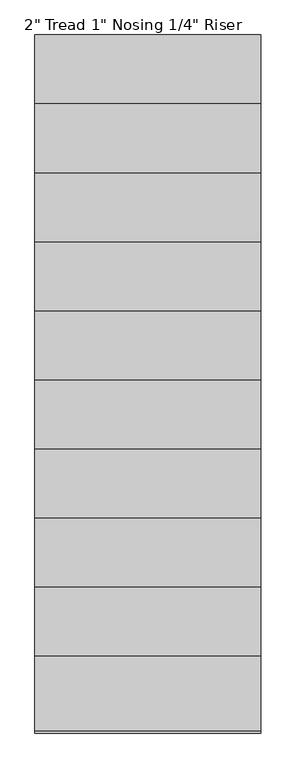
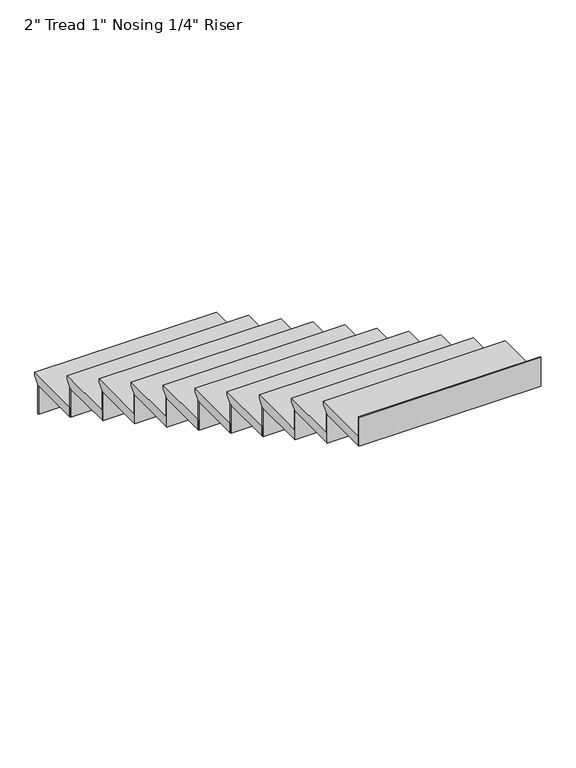
"""IFC4 building model written with IfcOpenShell, lengths in millimetres: stair flight geometry."""

from ifc_helpers import new_model, si_unit, frame, origin, place, context, project, spatial, polyline, outline, extrude, source, transform, mapped, element, save


def stair_flight_b2a94bac(model_context):
    return source(origin(), model_context, "Body", "SweptSolid", [
        extrude(outline(polyline([(4154.8726898, 1524.0), (4459.6726898, 1524.0), (4459.6726898, 1504.95), (4434.2726898, 1479.55), (4434.2726898, 1473.2), (4154.8726898, 1473.2), (4154.8726898, 1524.0)])), frame((1247.5463194, 0.0, 0.0), z_axis=(1.0, 0.0, 0.0), x_axis=(0.0, 1.0, 0.0)), (0.0, 0.0, 1.0), 914.4),
        extrude(outline(polyline([(1247.5463194, 4427.9226898), (1247.5463194, 4434.2726898), (2161.9463194, 4434.2726898), (2161.9463194, 4427.9226898), (1247.5463194, 4427.9226898)])), frame((0.0, 0.0, 1320.8), z_axis=(0.0, 0.0, 1.0), x_axis=(1.0, 0.0, 0.0)), (0.0, 0.0, 1.0), 152.4),
        extrude(outline(polyline([(1247.5463194, 4148.5226898), (1247.5463194, 4154.8726898), (2161.9463194, 4154.8726898), (2161.9463194, 4148.5226898), (1247.5463194, 4148.5226898)])), frame((0.0, 0.0, 1473.2), z_axis=(0.0, 0.0, 1.0), x_axis=(1.0, 0.0, 0.0)), (0.0, 0.0, 1.0), 152.4),
        extrude(outline(polyline([(3875.4726898, 1676.4), (4180.2726898, 1676.4), (4180.2726898, 1657.35), (4154.8726898, 1631.95), (4154.8726898, 1625.6), (3875.4726898, 1625.6), (3875.4726898, 1676.4)])), frame((1247.5463194, 0.0, 0.0), z_axis=(1.0, 0.0, 0.0), x_axis=(0.0, 1.0, 0.0)), (0.0, 0.0, 1.0), 914.4),
        extrude(outline(polyline([(1247.5463194, 3869.1226898), (1247.5463194, 3875.4726898), (2161.9463194, 3875.4726898), (2161.9463194, 3869.1226898), (1247.5463194, 3869.1226898)])), frame((0.0, 0.0, 1625.6), z_axis=(0.0, 0.0, 1.0), x_axis=(1.0, 0.0, 0.0)), (0.0, 0.0, 1.0), 152.4),
        extrude(outline(polyline([(3596.0726898, 1828.8), (3900.8726898, 1828.8), (3900.8726898, 1809.75), (3875.4726898, 1784.35), (3875.4726898, 1778.0), (3596.0726898, 1778.0), (3596.0726898, 1828.8)])), frame((1247.5463194, 0.0, 0.0), z_axis=(1.0, 0.0, 0.0), x_axis=(0.0, 1.0, 0.0)), (0.0, 0.0, 1.0), 914.4),
        extrude(outline(polyline([(1247.5463194, 3589.7226898), (1247.5463194, 3596.0726898), (2161.9463194, 3596.0726898), (2161.9463194, 3589.7226898), (1247.5463194, 3589.7226898)])), frame((0.0, 0.0, 1778.0), z_axis=(0.0, 0.0, 1.0), x_axis=(1.0, 0.0, 0.0)), (0.0, 0.0, 1.0), 152.4),
        extrude(outline(polyline([(3316.6726898, 1981.2), (3621.4726898, 1981.2), (3621.4726898, 1962.15), (3596.0726898, 1936.75), (3596.0726898, 1930.4), (3316.6726898, 1930.4), (3316.6726898, 1981.2)])), frame((1247.5463194, 0.0, 0.0), z_axis=(1.0, 0.0, 0.0), x_axis=(0.0, 1.0, 0.0)), (0.0, 0.0, 1.0), 914.4),
        extrude(outline(polyline([(1247.5463194, 3310.3226898), (1247.5463194, 3316.6726898), (2161.9463194, 3316.6726898), (2161.9463194, 3310.3226898), (1247.5463194, 3310.3226898)])), frame((0.0, 0.0, 1930.4), z_axis=(0.0, 0.0, 1.0), x_axis=(1.0, 0.0, 0.0)), (0.0, 0.0, 1.0), 152.4),
        extrude(outline(polyline([(3037.2726898, 2133.6), (3342.0726898, 2133.6), (3342.0726898, 2114.55), (3316.6726898, 2089.15), (3316.6726898, 2082.8), (3037.2726898, 2082.8), (3037.2726898, 2133.6)])), frame((1247.5463194, 0.0, 0.0), z_axis=(1.0, 0.0, 0.0), x_axis=(0.0, 1.0, 0.0)), (0.0, 0.0, 1.0), 914.4),
        extrude(outline(polyline([(1247.5463194, 3030.9226898), (1247.5463194, 3037.2726898), (2161.9463194, 3037.2726898), (2161.9463194, 3030.9226898), (1247.5463194, 3030.9226898)])), frame((0.0, 0.0, 2082.8), z_axis=(0.0, 0.0, 1.0), x_axis=(1.0, 0.0, 0.0)), (0.0, 0.0, 1.0), 152.4),
        extrude(outline(polyline([(2757.8726898, 2286.0), (3062.6726898, 2286.0), (3062.6726898, 2266.95), (3037.2726898, 2241.55), (3037.2726898, 2235.2), (2757.8726898, 2235.2), (2757.8726898, 2286.0)])), frame((1247.5463194, 0.0, 0.0), z_axis=(1.0, 0.0, 0.0), x_axis=(0.0, 1.0, 0.0)), (0.0, 0.0, 1.0), 914.4),
        extrude(outline(polyline([(1247.5463194, 2751.5226898), (1247.5463194, 2757.8726898), (2161.9463194, 2757.8726898), (2161.9463194, 2751.5226898), (1247.5463194, 2751.5226898)])), frame((0.0, 0.0, 2235.2), z_axis=(0.0, 0.0, 1.0), x_axis=(1.0, 0.0, 0.0)), (0.0, 0.0, 1.0), 152.4),
        extrude(outline(polyline([(2478.4726898, 2438.4), (2783.2726898, 2438.4), (2783.2726898, 2419.35), (2757.8726898, 2393.95), (2757.8726898, 2387.6), (2478.4726898, 2387.6), (2478.4726898, 2438.4)])), frame((1247.5463194, 0.0, 0.0), z_axis=(1.0, 0.0, 0.0), x_axis=(0.0, 1.0, 0.0)), (0.0, 0.0, 1.0), 914.4),
        extrude(outline(polyline([(1247.5463194, 2472.1226898), (1247.5463194, 2478.4726898), (2161.9463194, 2478.4726898), (2161.9463194, 2472.1226898), (1247.5463194, 2472.1226898)])), frame((0.0, 0.0, 2387.6), z_axis=(0.0, 0.0, 1.0), x_axis=(1.0, 0.0, 0.0)), (0.0, 0.0, 1.0), 152.4),
        extrude(outline(polyline([(2199.0726898, 2590.8), (2503.8726898, 2590.8), (2503.8726898, 2571.75), (2478.4726898, 2546.35), (2478.4726898, 2540.0), (2199.0726898, 2540.0), (2199.0726898, 2590.8)])), frame((1247.5463194, 0.0, 0.0), z_axis=(1.0, 0.0, 0.0), x_axis=(0.0, 1.0, 0.0)), (0.0, 0.0, 1.0), 914.4),
        extrude(outline(polyline([(1247.5463194, 2192.7226898), (1247.5463194, 2199.0726898), (2161.9463194, 2199.0726898), (2161.9463194, 2192.7226898), (1247.5463194, 2192.7226898)])), frame((0.0, 0.0, 2540.0), z_axis=(0.0, 0.0, 1.0), x_axis=(1.0, 0.0, 0.0)), (0.0, 0.0, 1.0), 152.4),
        extrude(outline(polyline([(1919.6726898, 2743.2), (2224.4726898, 2743.2), (2224.4726898, 2724.15), (2199.0726898, 2698.75), (2199.0726898, 2692.4), (1919.6726898, 2692.4), (1919.6726898, 2743.2)])), frame((1247.5463194, 0.0, 0.0), z_axis=(1.0, 0.0, 0.0), x_axis=(0.0, 1.0, 0.0)), (0.0, 0.0, 1.0), 914.4),
        extrude(outline(polyline([(1247.5463194, 1913.3226898), (1247.5463194, 1919.6726898), (2161.9463194, 1919.6726898), (2161.9463194, 1913.3226898), (1247.5463194, 1913.3226898)])), frame((0.0, 0.0, 2692.4), z_axis=(0.0, 0.0, 1.0), x_axis=(1.0, 0.0, 0.0)), (0.0, 0.0, 1.0), 152.4),
        extrude(outline(polyline([(1247.5463194, 1633.9226898), (1247.5463194, 1640.2726898), (2161.9463194, 1640.2726898), (2161.9463194, 1633.9226898), (1247.5463194, 1633.9226898)])), frame((0.0, 0.0, 2844.8), z_axis=(0.0, 0.0, 1.0), x_axis=(1.0, 0.0, 0.0)), (0.0, 0.0, 1.0), 152.4),
        extrude(outline(polyline([(1640.2726898, 2895.6), (1945.0726898, 2895.6), (1945.0726898, 2876.55), (1919.6726898, 2851.15), (1919.6726898, 2844.8), (1640.2726898, 2844.8), (1640.2726898, 2895.6)])), frame((1247.5463194, 0.0, 0.0), z_axis=(1.0, 0.0, 0.0), x_axis=(0.0, 1.0, 0.0)), (0.0, 0.0, 1.0), 914.4),
    ])


if __name__ == "__main__":
    model = new_model("IFC4")
    model_context = context("Model", 3, world=origin())
    ifc_project = project(units=[si_unit("LENGTHUNIT", "METRE", prefix="MILLI")], contexts=[model_context])
    site = spatial("IfcSite", under=ifc_project)
    building = spatial("IfcBuilding", under=site)
    placement = place(None, origin())
    stair_flight_shape = stair_flight_b2a94bac(model_context)
    element("IfcStairFlight", 1, ObjectType="2\" Tread 1\" Nosing 1/4\" Riser", at=placement, inside=building, context=model_context, shape_type="MappedRepresentation", body=[
        mapped(stair_flight_shape, transform((0.0, 0.0, 0.0), x_axis=(1.0, 0.0, 0.0), y_axis=(0.0, 1.0, 0.0), z_axis=(0.0, 0.0, 1.0))),
    ])
    save(model, "model.ifc")
